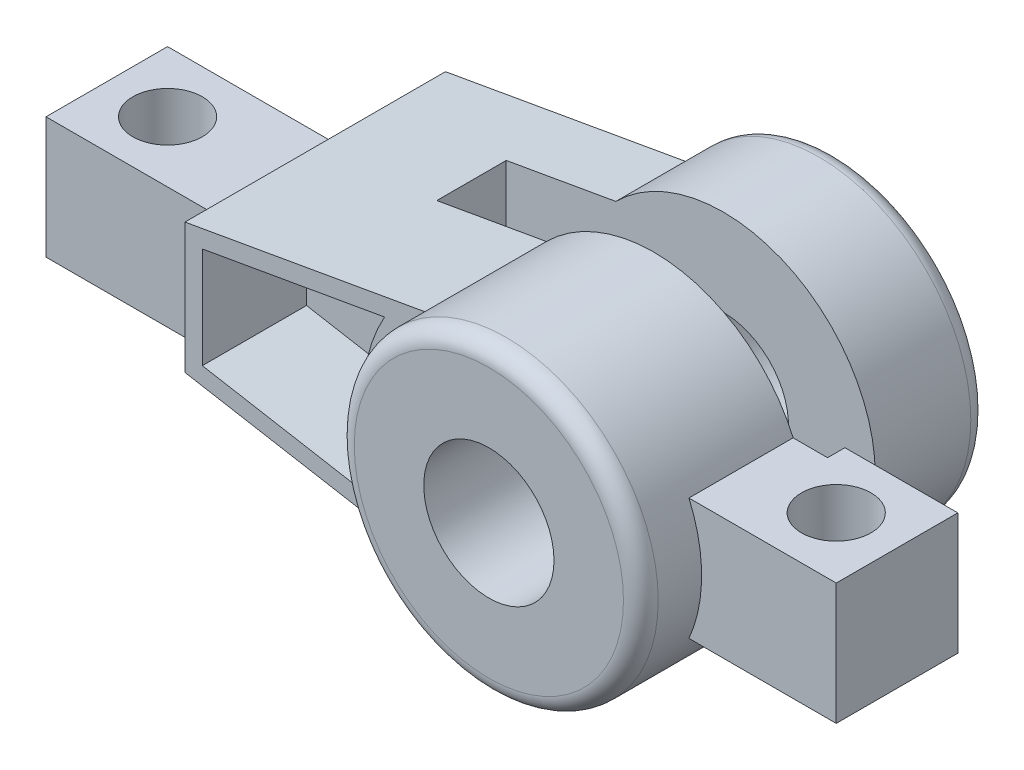
ISO-10303-21;
HEADER;
FILE_DESCRIPTION(('STEP AP214'),'2;1');
FILE_NAME('part.step','',(''),(''),'','','');
FILE_SCHEMA(('AUTOMOTIVE_DESIGN { 1 0 10303 214 1 1 1 1 }'));
ENDSEC;
DATA;
#1=APPLICATION_CONTEXT('core data for automotive mechanical design processes');
#2=APPLICATION_PROTOCOL_DEFINITION('international standard','automotive_design',2000,#1);
#3=PRODUCT_CONTEXT('',#1,'mechanical');
#4=PRODUCT('Part','Part','',(#3));
#5=PRODUCT_RELATED_PRODUCT_CATEGORY('part','',(#4));
#6=PRODUCT_DEFINITION_FORMATION('','',#4);
#7=PRODUCT_DEFINITION_CONTEXT('part definition',#1,'design');
#8=PRODUCT_DEFINITION('design','',#6,#7);
#9=PRODUCT_DEFINITION_SHAPE('','',#8);
#10=(LENGTH_UNIT() NAMED_UNIT(*) SI_UNIT(.MILLI.,.METRE.));
#11=(NAMED_UNIT(*) PLANE_ANGLE_UNIT() SI_UNIT($,.RADIAN.));
#12=(NAMED_UNIT(*) SI_UNIT($,.STERADIAN.) SOLID_ANGLE_UNIT());
#13=UNCERTAINTY_MEASURE_WITH_UNIT(LENGTH_MEASURE(1.E-05),#10,'distance_accuracy_value','');
#14=(GEOMETRIC_REPRESENTATION_CONTEXT(3) GLOBAL_UNCERTAINTY_ASSIGNED_CONTEXT((#13)) GLOBAL_UNIT_ASSIGNED_CONTEXT((#10,
#11,#12)) REPRESENTATION_CONTEXT('',''));
#15=CARTESIAN_POINT('',(0.,0.,0.));
#16=DIRECTION('',(0.,0.,1.));
#17=DIRECTION('',(1.,0.,0.));
#18=AXIS2_PLACEMENT_3D('',#15,#16,#17);
#19=CARTESIAN_POINT('',(46.,-6.99999999999998,20.));
#20=DIRECTION('',(0.,1.,0.));
#21=DIRECTION('',(-1.,0.,0.));
#22=AXIS2_PLACEMENT_3D('',#19,#20,#21);
#23=PLANE('',#22);
#24=CARTESIAN_POINT('',(39.,-6.99999999999998,6.));
#25=DIRECTION('',(0.,1.,0.));
#26=DIRECTION('',(-1.,0.,0.));
#27=AXIS2_PLACEMENT_3D('',#24,#25,#26);
#28=CIRCLE('',#27,5.);
#29=CARTESIAN_POINT('',(34.,-6.99999999999999,6.));
#30=VERTEX_POINT('',#29);
#31=EDGE_CURVE('E11',#30,#30,#28,.T.);
#32=ORIENTED_EDGE('',*,*,#31,.T.);
#33=EDGE_LOOP('',(#32));
#34=FACE_BOUND('',#33,.T.);
#35=DIRECTION('',(-1.,0.,0.));
#36=VECTOR('',#35,1.);
#37=CARTESIAN_POINT('',(46.,-6.99999999999998,-1.));
#38=LINE('',#37,#36);
#39=CARTESIAN_POINT('',(46.,-6.99999999999998,-1.));
#40=VERTEX_POINT('',#39);
#41=CARTESIAN_POINT('',(33.,-6.99999999999999,-1.));
#42=VERTEX_POINT('',#41);
#43=EDGE_CURVE('E293',#40,#42,#38,.T.);
#44=ORIENTED_EDGE('',*,*,#43,.F.);
#45=DIRECTION('',(0.,0.,-1.));
#46=VECTOR('',#45,1.);
#47=CARTESIAN_POINT('',(46.,-6.99999999999998,20.));
#48=LINE('',#47,#46);
#49=CARTESIAN_POINT('',(46.,-6.99999999999998,13.));
#50=VERTEX_POINT('',#49);
#51=EDGE_CURVE('E396',#50,#40,#48,.T.);
#52=ORIENTED_EDGE('',*,*,#51,.F.);
#53=DIRECTION('',(1.,0.,0.));
#54=VECTOR('',#53,1.);
#55=CARTESIAN_POINT('',(29.0390149323454,-6.99999999999998,13.));
#56=LINE('',#55,#54);
#57=CARTESIAN_POINT('',(29.0390149323454,-6.99999999999998,13.));
#58=VERTEX_POINT('',#57);
#59=EDGE_CURVE('E332',#58,#50,#56,.T.);
#60=ORIENTED_EDGE('',*,*,#59,.F.);
#61=DIRECTION('',(0.,0.,-1.));
#62=VECTOR('',#61,1.);
#63=CARTESIAN_POINT('',(29.0390149323454,-6.99999999999998,20.));
#64=LINE('',#63,#62);
#65=CARTESIAN_POINT('',(29.0390149323454,-6.99999999999999,1.));
#66=VERTEX_POINT('',#65);
#67=EDGE_CURVE('E397',#58,#66,#64,.T.);
#68=ORIENTED_EDGE('',*,*,#67,.T.);
#69=DIRECTION('',(1.,0.,0.));
#70=VECTOR('',#69,1.);
#71=CARTESIAN_POINT('',(46.,-6.99999999999998,1.));
#72=LINE('',#71,#70);
#73=CARTESIAN_POINT('',(33.,-6.99999999999999,1.));
#74=VERTEX_POINT('',#73);
#75=EDGE_CURVE('E363',#66,#74,#72,.T.);
#76=ORIENTED_EDGE('',*,*,#75,.T.);
#77=DIRECTION('',(0.,0.,-1.));
#78=VECTOR('',#77,1.);
#79=CARTESIAN_POINT('',(33.,-6.99999999999999,20.));
#80=LINE('',#79,#78);
#81=EDGE_CURVE('E379',#74,#42,#80,.T.);
#82=ORIENTED_EDGE('',*,*,#81,.T.);
#83=EDGE_LOOP('',(#44,#52,#60,#68,#76,#82));
#84=FACE_BOUND('',#83,.T.);
#85=ADVANCED_FACE('F41',(#34,#84),#23,.F.);
#86=CARTESIAN_POINT('',(46.,-6.99999999999998,20.));
#87=DIRECTION('',(-1.,0.,0.));
#88=DIRECTION('',(0.,0.,1.));
#89=AXIS2_PLACEMENT_3D('',#86,#87,#88);
#90=PLANE('',#89);
#91=DIRECTION('',(0.,-1.,0.));
#92=VECTOR('',#91,1.);
#93=CARTESIAN_POINT('',(46.,7.00000000000002,-1.));
#94=LINE('',#93,#92);
#95=CARTESIAN_POINT('',(46.,7.00000000000002,-1.));
#96=VERTEX_POINT('',#95);
#97=EDGE_CURVE('E288',#96,#40,#94,.T.);
#98=ORIENTED_EDGE('',*,*,#97,.F.);
#99=DIRECTION('',(0.,0.,-1.));
#100=VECTOR('',#99,1.);
#101=CARTESIAN_POINT('',(46.,7.00000000000002,20.));
#102=LINE('',#101,#100);
#103=CARTESIAN_POINT('',(46.,7.00000000000002,13.));
#104=VERTEX_POINT('',#103);
#105=EDGE_CURVE('E392',#104,#96,#102,.T.);
#106=ORIENTED_EDGE('',*,*,#105,.F.);
#107=DIRECTION('',(0.,1.,0.));
#108=VECTOR('',#107,1.);
#109=CARTESIAN_POINT('',(46.,-6.99999999999998,13.));
#110=LINE('',#109,#108);
#111=EDGE_CURVE('E340',#50,#104,#110,.T.);
#112=ORIENTED_EDGE('',*,*,#111,.F.);
#113=ORIENTED_EDGE('',*,*,#51,.T.);
#114=EDGE_LOOP('',(#98,#106,#112,#113));
#115=FACE_BOUND('',#114,.T.);
#116=ADVANCED_FACE('F457',(#115),#90,.F.);
#117=CARTESIAN_POINT('',(46.,7.00000000000002,20.));
#118=DIRECTION('',(0.,-1.,0.));
#119=DIRECTION('',(1.,0.,0.));
#120=AXIS2_PLACEMENT_3D('',#117,#118,#119);
#121=PLANE('',#120);
#122=CARTESIAN_POINT('',(39.,7.,6.));
#123=DIRECTION('',(0.,1.,0.));
#124=DIRECTION('',(-1.,0.,0.));
#125=AXIS2_PLACEMENT_3D('',#122,#123,#124);
#126=CIRCLE('',#125,4.);
#127=CARTESIAN_POINT('',(35.,7.,6.));
#128=VERTEX_POINT('',#127);
#129=EDGE_CURVE('E241',#128,#128,#126,.T.);
#130=ORIENTED_EDGE('',*,*,#129,.F.);
#131=EDGE_LOOP('',(#130));
#132=FACE_BOUND('',#131,.T.);
#133=DIRECTION('',(1.,0.,0.));
#134=VECTOR('',#133,1.);
#135=CARTESIAN_POINT('',(29.0390149323454,7.00000000000001,-1.));
#136=LINE('',#135,#134);
#137=CARTESIAN_POINT('',(33.,7.00000000000002,-1.));
#138=VERTEX_POINT('',#137);
#139=EDGE_CURVE('E285',#138,#96,#136,.T.);
#140=ORIENTED_EDGE('',*,*,#139,.F.);
#141=DIRECTION('',(0.,0.,1.));
#142=VECTOR('',#141,1.);
#143=CARTESIAN_POINT('',(33.,7.00000000000002,20.));
#144=LINE('',#143,#142);
#145=CARTESIAN_POINT('',(33.,7.00000000000002,1.));
#146=VERTEX_POINT('',#145);
#147=EDGE_CURVE('E422',#138,#146,#144,.T.);
#148=ORIENTED_EDGE('',*,*,#147,.T.);
#149=DIRECTION('',(-1.,0.,0.));
#150=VECTOR('',#149,1.);
#151=CARTESIAN_POINT('',(46.,7.00000000000002,1.));
#152=LINE('',#151,#150);
#153=CARTESIAN_POINT('',(29.0390149323454,7.00000000000001,1.));
#154=VERTEX_POINT('',#153);
#155=EDGE_CURVE('E351',#146,#154,#152,.T.);
#156=ORIENTED_EDGE('',*,*,#155,.T.);
#157=DIRECTION('',(0.,0.,-1.));
#158=VECTOR('',#157,1.);
#159=CARTESIAN_POINT('',(29.0390149323454,7.00000000000001,20.));
#160=LINE('',#159,#158);
#161=CARTESIAN_POINT('',(29.0390149323454,7.00000000000001,13.));
#162=VERTEX_POINT('',#161);
#163=EDGE_CURVE('E388',#162,#154,#160,.T.);
#164=ORIENTED_EDGE('',*,*,#163,.F.);
#165=DIRECTION('',(-1.,0.,0.));
#166=VECTOR('',#165,1.);
#167=CARTESIAN_POINT('',(46.,7.00000000000002,13.));
#168=LINE('',#167,#166);
#169=EDGE_CURVE('E339',#104,#162,#168,.T.);
#170=ORIENTED_EDGE('',*,*,#169,.F.);
#171=ORIENTED_EDGE('',*,*,#105,.T.);
#172=EDGE_LOOP('',(#140,#148,#156,#164,#170,#171));
#173=FACE_BOUND('',#172,.T.);
#174=ADVANCED_FACE('F467',(#132,#173),#121,.F.);
#175=CARTESIAN_POINT('',(33.,-17.5,-7.));
#176=DIRECTION('',(1.,0.,0.));
#177=DIRECTION('',(0.,0.,-1.));
#178=AXIS2_PLACEMENT_3D('',#175,#176,#177);
#179=PLANE('',#178);
#180=DIRECTION('',(0.,1.,0.));
#181=VECTOR('',#180,1.);
#182=CARTESIAN_POINT('',(33.,-17.5,-1.));
#183=LINE('',#182,#181);
#184=EDGE_CURVE('E431',#42,#138,#183,.T.);
#185=ORIENTED_EDGE('',*,*,#184,.F.);
#186=ORIENTED_EDGE('',*,*,#81,.F.);
#187=DIRECTION('',(0.,1.,0.));
#188=VECTOR('',#187,1.);
#189=CARTESIAN_POINT('',(33.,-17.5,1.));
#190=LINE('',#189,#188);
#191=EDGE_CURVE('E350',#74,#146,#190,.T.);
#192=ORIENTED_EDGE('',*,*,#191,.T.);
#193=ORIENTED_EDGE('',*,*,#147,.F.);
#194=EDGE_LOOP('',(#185,#186,#192,#193));
#195=FACE_BOUND('',#194,.T.);
#196=ADVANCED_FACE('F499',(#195),#179,.F.);
#197=CARTESIAN_POINT('',(-46.,7.,20.));
#198=DIRECTION('',(0.,-1.,0.));
#199=DIRECTION('',(1.,0.,0.));
#200=AXIS2_PLACEMENT_3D('',#197,#198,#199);
#201=PLANE('',#200);
#202=CARTESIAN_POINT('',(-39.,7.,5.));
#203=DIRECTION('',(0.,1.,0.));
#204=DIRECTION('',(-1.,0.,0.));
#205=AXIS2_PLACEMENT_3D('',#202,#203,#204);
#206=CIRCLE('',#205,4.);
#207=CARTESIAN_POINT('',(-43.,7.,5.));
#208=VERTEX_POINT('',#207);
#209=EDGE_CURVE('E944',#208,#208,#206,.T.);
#210=ORIENTED_EDGE('',*,*,#209,.F.);
#211=EDGE_LOOP('',(#210));
#212=FACE_BOUND('',#211,.T.);
#213=DIRECTION('',(-1.,0.,0.));
#214=VECTOR('',#213,1.);
#215=CARTESIAN_POINT('',(-27.,7.,12.));
#216=LINE('',#215,#214);
#217=CARTESIAN_POINT('',(-27.,7.,12.));
#218=VERTEX_POINT('',#217);
#219=CARTESIAN_POINT('',(-46.,7.,12.));
#220=VERTEX_POINT('',#219);
#221=EDGE_CURVE('E294',#218,#220,#216,.T.);
#222=ORIENTED_EDGE('',*,*,#221,.F.);
#223=DIRECTION('',(0.,0.,-1.));
#224=VECTOR('',#223,1.);
#225=CARTESIAN_POINT('',(-27.,7.,20.));
#226=LINE('',#225,#224);
#227=CARTESIAN_POINT('',(-27.,7.,-2.));
#228=VERTEX_POINT('',#227);
#229=EDGE_CURVE('E412',#218,#228,#226,.T.);
#230=ORIENTED_EDGE('',*,*,#229,.T.);
#231=DIRECTION('',(1.,0.,0.));
#232=VECTOR('',#231,1.);
#233=CARTESIAN_POINT('',(-46.,7.,-2.));
#234=LINE('',#233,#232);
#235=CARTESIAN_POINT('',(-46.,7.,-2.));
#236=VERTEX_POINT('',#235);
#237=EDGE_CURVE('E304',#236,#228,#234,.T.);
#238=ORIENTED_EDGE('',*,*,#237,.F.);
#239=DIRECTION('',(0.,0.,-1.));
#240=VECTOR('',#239,1.);
#241=CARTESIAN_POINT('',(-46.,7.,20.));
#242=LINE('',#241,#240);
#243=EDGE_CURVE('E415',#220,#236,#242,.T.);
#244=ORIENTED_EDGE('',*,*,#243,.F.);
#245=EDGE_LOOP('',(#222,#230,#238,#244));
#246=FACE_BOUND('',#245,.T.);
#247=ADVANCED_FACE('F496',(#212,#246),#201,.F.);
#248=CARTESIAN_POINT('',(-46.,-7.,20.));
#249=DIRECTION('',(1.,0.,0.));
#250=DIRECTION('',(0.,0.,-1.));
#251=AXIS2_PLACEMENT_3D('',#248,#249,#250);
#252=PLANE('',#251);
#253=DIRECTION('',(0.,-1.,0.));
#254=VECTOR('',#253,1.);
#255=CARTESIAN_POINT('',(-46.,7.,12.));
#256=LINE('',#255,#254);
#257=CARTESIAN_POINT('',(-46.,-7.,12.));
#258=VERTEX_POINT('',#257);
#259=EDGE_CURVE('E300',#220,#258,#256,.T.);
#260=ORIENTED_EDGE('',*,*,#259,.F.);
#261=ORIENTED_EDGE('',*,*,#243,.T.);
#262=DIRECTION('',(0.,1.,0.));
#263=VECTOR('',#262,1.);
#264=CARTESIAN_POINT('',(-46.,-7.,-2.));
#265=LINE('',#264,#263);
#266=CARTESIAN_POINT('',(-46.,-7.,-2.));
#267=VERTEX_POINT('',#266);
#268=EDGE_CURVE('E305',#267,#236,#265,.T.);
#269=ORIENTED_EDGE('',*,*,#268,.F.);
#270=DIRECTION('',(0.,0.,-1.));
#271=VECTOR('',#270,1.);
#272=CARTESIAN_POINT('',(-46.,-7.,20.));
#273=LINE('',#272,#271);
#274=EDGE_CURVE('E408',#258,#267,#273,.T.);
#275=ORIENTED_EDGE('',*,*,#274,.F.);
#276=EDGE_LOOP('',(#260,#261,#269,#275));
#277=FACE_BOUND('',#276,.T.);
#278=ADVANCED_FACE('F495',(#277),#252,.F.);
#279=CARTESIAN_POINT('',(-46.,-7.,20.));
#280=DIRECTION('',(0.,1.,0.));
#281=DIRECTION('',(-1.,0.,0.));
#282=AXIS2_PLACEMENT_3D('',#279,#280,#281);
#283=PLANE('',#282);
#284=CARTESIAN_POINT('',(-39.,-7.,5.));
#285=DIRECTION('',(0.,1.,0.));
#286=DIRECTION('',(-1.,0.,0.));
#287=AXIS2_PLACEMENT_3D('',#284,#285,#286);
#288=CIRCLE('',#287,4.);
#289=CARTESIAN_POINT('',(-43.,-7.,5.));
#290=VERTEX_POINT('',#289);
#291=EDGE_CURVE('E247',#290,#290,#288,.F.);
#292=ORIENTED_EDGE('',*,*,#291,.F.);
#293=EDGE_LOOP('',(#292));
#294=FACE_BOUND('',#293,.T.);
#295=DIRECTION('',(1.,0.,0.));
#296=VECTOR('',#295,1.);
#297=CARTESIAN_POINT('',(-46.,-7.,12.));
#298=LINE('',#297,#296);
#299=CARTESIAN_POINT('',(-27.,-6.99999999999999,12.));
#300=VERTEX_POINT('',#299);
#301=EDGE_CURVE('E299',#258,#300,#298,.T.);
#302=ORIENTED_EDGE('',*,*,#301,.F.);
#303=ORIENTED_EDGE('',*,*,#274,.T.);
#304=DIRECTION('',(-1.,0.,0.));
#305=VECTOR('',#304,1.);
#306=CARTESIAN_POINT('',(-27.,-6.99999999999999,-2.));
#307=LINE('',#306,#305);
#308=CARTESIAN_POINT('',(-27.,-6.99999999999999,-2.));
#309=VERTEX_POINT('',#308);
#310=EDGE_CURVE('E311',#309,#267,#307,.T.);
#311=ORIENTED_EDGE('',*,*,#310,.F.);
#312=DIRECTION('',(0.,0.,-1.));
#313=VECTOR('',#312,1.);
#314=CARTESIAN_POINT('',(-27.,-6.99999999999999,20.));
#315=LINE('',#314,#313);
#316=EDGE_CURVE('E409',#300,#309,#315,.T.);
#317=ORIENTED_EDGE('',*,*,#316,.F.);
#318=EDGE_LOOP('',(#302,#303,#311,#317));
#319=FACE_BOUND('',#318,.T.);
#320=ADVANCED_FACE('F490',(#294,#319),#283,.F.);
#321=CARTESIAN_POINT('',(-27.,7.5,20.));
#322=DIRECTION('',(0.173648177666928,-0.984807753012209,0.));
#323=DIRECTION('',(0.984807753012209,0.173648177666928,0.));
#324=AXIS2_PLACEMENT_3D('',#321,#322,#323);
#325=PLANE('',#324);
#326=DIRECTION('',(0.984807753012209,0.173648177666928,0.));
#327=VECTOR('',#326,1.);
#328=CARTESIAN_POINT('',(0.621718040461723,12.3704541440551,-15.));
#329=LINE('',#328,#327);
#330=CARTESIAN_POINT('',(-27.,7.5,-15.));
#331=VERTEX_POINT('',#330);
#332=CARTESIAN_POINT('',(0.621718040461723,12.3704541440551,-15.));
#333=VERTEX_POINT('',#332);
#334=EDGE_CURVE('E322',#331,#333,#329,.T.);
#335=ORIENTED_EDGE('',*,*,#334,.F.);
#336=DIRECTION('',(0.,0.,-1.));
#337=VECTOR('',#336,1.);
#338=CARTESIAN_POINT('',(-27.,7.5,20.));
#339=LINE('',#338,#337);
#340=CARTESIAN_POINT('',(-27.,7.5,15.));
#341=VERTEX_POINT('',#340);
#342=EDGE_CURVE('E419',#341,#331,#339,.T.);
#343=ORIENTED_EDGE('',*,*,#342,.F.);
#344=DIRECTION('',(-0.984807753012209,-0.173648177666928,0.));
#345=VECTOR('',#344,1.);
#346=CARTESIAN_POINT('',(-2.09672515686145,11.8911192628436,15.));
#347=LINE('',#346,#345);
#348=CARTESIAN_POINT('',(0.621718040461722,12.3704541440551,15.));
#349=VERTEX_POINT('',#348);
#350=EDGE_CURVE('E326',#349,#341,#347,.T.);
#351=ORIENTED_EDGE('',*,*,#350,.F.);
#352=DIRECTION('',(0.,0.,-1.));
#353=VECTOR('',#352,1.);
#354=CARTESIAN_POINT('',(0.621718040461723,12.3704541440551,20.));
#355=LINE('',#354,#353);
#356=CARTESIAN_POINT('',(0.621718040461723,12.3704541440551,1.));
#357=VERTEX_POINT('',#356);
#358=EDGE_CURVE('E417',#349,#357,#355,.T.);
#359=ORIENTED_EDGE('',*,*,#358,.T.);
#360=DIRECTION('',(-0.984807753012209,-0.173648177666928,0.));
#361=VECTOR('',#360,1.);
#362=CARTESIAN_POINT('',(-27.,7.5,1.));
#363=LINE('',#362,#361);
#364=CARTESIAN_POINT('',(-12.,10.1449047106269,1.));
#365=VERTEX_POINT('',#364);
#366=EDGE_CURVE('E356',#357,#365,#363,.T.);
#367=ORIENTED_EDGE('',*,*,#366,.T.);
#368=DIRECTION('',(0.,0.,-1.));
#369=VECTOR('',#368,1.);
#370=CARTESIAN_POINT('',(-12.,10.1449047106269,20.));
#371=LINE('',#370,#369);
#372=CARTESIAN_POINT('',(-12.,10.1449047106269,-7.));
#373=VERTEX_POINT('',#372);
#374=EDGE_CURVE('E384',#365,#373,#371,.T.);
#375=ORIENTED_EDGE('',*,*,#374,.T.);
#376=DIRECTION('',(0.984807753012209,0.173648177666928,0.));
#377=VECTOR('',#376,1.);
#378=CARTESIAN_POINT('',(-27.,7.5,-7.));
#379=LINE('',#378,#377);
#380=CARTESIAN_POINT('',(0.621718040461723,12.3704541440551,-7.));
#381=VERTEX_POINT('',#380);
#382=EDGE_CURVE('E371',#373,#381,#379,.T.);
#383=ORIENTED_EDGE('',*,*,#382,.T.);
#384=EDGE_CURVE('E418',#381,#333,#355,.T.);
#385=ORIENTED_EDGE('',*,*,#384,.T.);
#386=EDGE_LOOP('',(#335,#343,#351,#359,#367,#375,#383,#385));
#387=FACE_BOUND('',#386,.T.);
#388=ADVANCED_FACE('F487',(#387),#325,.F.);
#389=CARTESIAN_POINT('',(-27.,-6.99999999999999,20.));
#390=DIRECTION('',(1.,0.,0.));
#391=DIRECTION('',(0.,0.,-1.));
#392=AXIS2_PLACEMENT_3D('',#389,#390,#391);
#393=PLANE('',#392);
#394=DIRECTION('',(0.,1.,0.));
#395=VECTOR('',#394,1.);
#396=CARTESIAN_POINT('',(-27.,-6.99999999999999,12.));
#397=LINE('',#396,#395);
#398=EDGE_CURVE('E291',#300,#218,#397,.T.);
#399=ORIENTED_EDGE('',*,*,#398,.F.);
#400=ORIENTED_EDGE('',*,*,#316,.T.);
#401=DIRECTION('',(0.,-1.,0.));
#402=VECTOR('',#401,1.);
#403=CARTESIAN_POINT('',(-27.,7.,-2.));
#404=LINE('',#403,#402);
#405=EDGE_CURVE('E308',#228,#309,#404,.T.);
#406=ORIENTED_EDGE('',*,*,#405,.F.);
#407=ORIENTED_EDGE('',*,*,#229,.F.);
#408=EDGE_LOOP('',(#399,#400,#406,#407));
#409=FACE_BOUND('',#408,.T.);
#410=ORIENTED_EDGE('',*,*,#342,.T.);
#411=DIRECTION('',(0.,1.,0.));
#412=VECTOR('',#411,1.);
#413=CARTESIAN_POINT('',(-27.,7.5,-15.));
#414=LINE('',#413,#412);
#415=CARTESIAN_POINT('',(-27.,-7.49999999999999,-15.));
#416=VERTEX_POINT('',#415);
#417=EDGE_CURVE('E316',#416,#331,#414,.T.);
#418=ORIENTED_EDGE('',*,*,#417,.F.);
#419=DIRECTION('',(0.,0.,-1.));
#420=VECTOR('',#419,1.);
#421=CARTESIAN_POINT('',(-27.,-7.49999999999999,20.));
#422=LINE('',#421,#420);
#423=CARTESIAN_POINT('',(-27.,-7.49999999999999,15.));
#424=VERTEX_POINT('',#423);
#425=EDGE_CURVE('E403',#424,#416,#422,.T.);
#426=ORIENTED_EDGE('',*,*,#425,.F.);
#427=DIRECTION('',(0.,-1.,0.));
#428=VECTOR('',#427,1.);
#429=CARTESIAN_POINT('',(-27.,0.,15.));
#430=LINE('',#429,#428);
#431=EDGE_CURVE('E328',#341,#424,#430,.T.);
#432=ORIENTED_EDGE('',*,*,#431,.F.);
#433=EDGE_LOOP('',(#410,#418,#426,#432));
#434=FACE_BOUND('',#433,.T.);
#435=ADVANCED_FACE('F485',(#409,#434),#393,.F.);
#436=CARTESIAN_POINT('',(-27.,-7.49999999999999,20.));
#437=DIRECTION('',(0.173648177666927,0.984807753012209,0.));
#438=DIRECTION('',(-0.984807753012209,0.173648177666927,0.));
#439=AXIS2_PLACEMENT_3D('',#436,#437,#438);
#440=PLANE('',#439);
#441=DIRECTION('',(-0.984807753012209,0.173648177666927,0.));
#442=VECTOR('',#441,1.);
#443=CARTESIAN_POINT('',(-27.,-7.49999999999999,-15.));
#444=LINE('',#443,#442);
#445=CARTESIAN_POINT('',(0.621718040461723,-12.3704541440551,-15.));
#446=VERTEX_POINT('',#445);
#447=EDGE_CURVE('E317',#446,#416,#444,.T.);
#448=ORIENTED_EDGE('',*,*,#447,.F.);
#449=DIRECTION('',(0.,0.,-1.));
#450=VECTOR('',#449,1.);
#451=CARTESIAN_POINT('',(0.621718040461723,-12.3704541440551,20.));
#452=LINE('',#451,#450);
#453=CARTESIAN_POINT('',(0.621718040461719,-12.3704541440551,-7.));
#454=VERTEX_POINT('',#453);
#455=EDGE_CURVE('E405',#454,#446,#452,.T.);
#456=ORIENTED_EDGE('',*,*,#455,.F.);
#457=DIRECTION('',(-0.984807753012209,0.173648177666927,0.));
#458=VECTOR('',#457,1.);
#459=CARTESIAN_POINT('',(-27.,-7.49999999999999,-7.));
#460=LINE('',#459,#458);
#461=CARTESIAN_POINT('',(-12.,-10.1449047106269,-7.));
#462=VERTEX_POINT('',#461);
#463=EDGE_CURVE('E380',#454,#462,#460,.T.);
#464=ORIENTED_EDGE('',*,*,#463,.T.);
#465=DIRECTION('',(0.,0.,1.));
#466=VECTOR('',#465,1.);
#467=CARTESIAN_POINT('',(-12.,-10.1449047106269,20.));
#468=LINE('',#467,#466);
#469=CARTESIAN_POINT('',(-12.,-10.1449047106269,1.));
#470=VERTEX_POINT('',#469);
#471=EDGE_CURVE('E426',#462,#470,#468,.T.);
#472=ORIENTED_EDGE('',*,*,#471,.T.);
#473=DIRECTION('',(0.984807753012209,-0.173648177666927,0.));
#474=VECTOR('',#473,1.);
#475=CARTESIAN_POINT('',(-27.,-7.49999999999999,1.));
#476=LINE('',#475,#474);
#477=CARTESIAN_POINT('',(0.621718040461719,-12.3704541440551,1.));
#478=VERTEX_POINT('',#477);
#479=EDGE_CURVE('E370',#470,#478,#476,.T.);
#480=ORIENTED_EDGE('',*,*,#479,.T.);
#481=CARTESIAN_POINT('',(0.621718040461711,-12.3704541440551,15.));
#482=VERTEX_POINT('',#481);
#483=EDGE_CURVE('E401',#482,#478,#452,.T.);
#484=ORIENTED_EDGE('',*,*,#483,.F.);
#485=DIRECTION('',(0.984807753012209,-0.173648177666927,0.));
#486=VECTOR('',#485,1.);
#487=CARTESIAN_POINT('',(-2.09672515686144,-11.8911192628436,15.));
#488=LINE('',#487,#486);
#489=EDGE_CURVE('E329',#424,#482,#488,.T.);
#490=ORIENTED_EDGE('',*,*,#489,.F.);
#491=ORIENTED_EDGE('',*,*,#425,.T.);
#492=EDGE_LOOP('',(#448,#456,#464,#472,#480,#484,#490,#491));
#493=FACE_BOUND('',#492,.T.);
#494=ADVANCED_FACE('F477',(#493),#440,.F.);
#495=CARTESIAN_POINT('',(13.,0.,-20.));
#496=DIRECTION('',(0.,0.,1.));
#497=DIRECTION('',(1.,0.,0.));
#498=AXIS2_PLACEMENT_3D('',#495,#496,#497);
#499=PLANE('',#498);
#500=CARTESIAN_POINT('',(13.,0.,-20.));
#501=DIRECTION('',(0.,0.,1.));
#502=DIRECTION('',(1.,0.,0.));
#503=AXIS2_PLACEMENT_3D('',#500,#501,#502);
#504=CIRCLE('',#503,15.5);
#505=CARTESIAN_POINT('',(28.5,0.,-20.));
#506=VERTEX_POINT('',#505);
#507=EDGE_CURVE('E445',#506,#506,#504,.F.);
#508=ORIENTED_EDGE('',*,*,#507,.T.);
#509=EDGE_LOOP('',(#508));
#510=FACE_BOUND('',#509,.T.);
#511=CARTESIAN_POINT('',(13.,0.,-20.));
#512=DIRECTION('',(0.,0.,1.));
#513=DIRECTION('',(1.,0.,0.));
#514=AXIS2_PLACEMENT_3D('',#511,#512,#513);
#515=CIRCLE('',#514,7.5);
#516=CARTESIAN_POINT('',(20.5,0.,-20.));
#517=VERTEX_POINT('',#516);
#518=EDGE_CURVE('E387',#517,#517,#515,.T.);
#519=ORIENTED_EDGE('',*,*,#518,.T.);
#520=EDGE_LOOP('',(#519));
#521=FACE_BOUND('',#520,.T.);
#522=ADVANCED_FACE('F481',(#510,#521),#499,.F.);
#523=CARTESIAN_POINT('',(13.,0.,20.));
#524=DIRECTION('',(0.,0.,1.));
#525=DIRECTION('',(1.,0.,0.));
#526=AXIS2_PLACEMENT_3D('',#523,#524,#525);
#527=PLANE('',#526);
#528=CARTESIAN_POINT('',(13.,0.,20.));
#529=DIRECTION('',(0.,0.,1.));
#530=DIRECTION('',(1.,0.,0.));
#531=AXIS2_PLACEMENT_3D('',#528,#529,#530);
#532=CIRCLE('',#531,15.5);
#533=CARTESIAN_POINT('',(28.5,0.,20.));
#534=VERTEX_POINT('',#533);
#535=EDGE_CURVE('E433',#534,#534,#532,.T.);
#536=ORIENTED_EDGE('',*,*,#535,.T.);
#537=EDGE_LOOP('',(#536));
#538=FACE_BOUND('',#537,.T.);
#539=CARTESIAN_POINT('',(13.,0.,20.));
#540=DIRECTION('',(0.,0.,1.));
#541=DIRECTION('',(1.,0.,0.));
#542=AXIS2_PLACEMENT_3D('',#539,#540,#541);
#543=CIRCLE('',#542,7.5);
#544=CARTESIAN_POINT('',(20.5,0.,20.));
#545=VERTEX_POINT('',#544);
#546=EDGE_CURVE('E390',#545,#545,#543,.T.);
#547=ORIENTED_EDGE('',*,*,#546,.F.);
#548=EDGE_LOOP('',(#547));
#549=FACE_BOUND('',#548,.T.);
#550=ADVANCED_FACE('F583',(#538,#549),#527,.T.);
#551=CARTESIAN_POINT('',(13.,0.,20.));
#552=DIRECTION('',(0.,0.,-1.));
#553=DIRECTION('',(-1.,0.,0.));
#554=AXIS2_PLACEMENT_3D('',#551,#552,#553);
#555=CYLINDRICAL_SURFACE('',#554,17.5);
#556=CARTESIAN_POINT('',(13.,0.,18.));
#557=DIRECTION('',(0.,0.,1.));
#558=DIRECTION('',(1.,0.,0.));
#559=AXIS2_PLACEMENT_3D('',#556,#557,#558);
#560=CIRCLE('',#559,17.5);
#561=CARTESIAN_POINT('',(30.5,0.,18.));
#562=VERTEX_POINT('',#561);
#563=EDGE_CURVE('E436',#562,#562,#560,.F.);
#564=ORIENTED_EDGE('',*,*,#563,.T.);
#565=EDGE_LOOP('',(#564));
#566=FACE_BOUND('',#565,.T.);
#567=ORIENTED_EDGE('',*,*,#358,.F.);
#568=CARTESIAN_POINT('',(13.,0.,15.));
#569=DIRECTION('',(0.,0.,1.));
#570=DIRECTION('',(1.,0.,0.));
#571=AXIS2_PLACEMENT_3D('',#568,#569,#570);
#572=CIRCLE('',#571,17.5);
#573=EDGE_CURVE('E321',#349,#482,#572,.T.);
#574=ORIENTED_EDGE('',*,*,#573,.T.);
#575=ORIENTED_EDGE('',*,*,#483,.T.);
#576=CARTESIAN_POINT('',(13.,0.,1.));
#577=DIRECTION('',(0.,0.,1.));
#578=DIRECTION('',(1.,0.,0.));
#579=AXIS2_PLACEMENT_3D('',#576,#577,#578);
#580=CIRCLE('',#579,17.5);
#581=EDGE_CURVE('E364',#478,#66,#580,.T.);
#582=ORIENTED_EDGE('',*,*,#581,.T.);
#583=ORIENTED_EDGE('',*,*,#67,.F.);
#584=CARTESIAN_POINT('',(13.,0.,13.));
#585=DIRECTION('',(0.,0.,-1.));
#586=DIRECTION('',(1.,0.,0.));
#587=AXIS2_PLACEMENT_3D('',#584,#585,#586);
#588=CIRCLE('',#587,17.5);
#589=EDGE_CURVE('E335',#162,#58,#588,.T.);
#590=ORIENTED_EDGE('',*,*,#589,.F.);
#591=ORIENTED_EDGE('',*,*,#163,.T.);
#592=CARTESIAN_POINT('',(13.,0.,1.));
#593=DIRECTION('',(0.,0.,1.));
#594=DIRECTION('',(1.,0.,0.));
#595=AXIS2_PLACEMENT_3D('',#592,#593,#594);
#596=CIRCLE('',#595,17.5);
#597=EDGE_CURVE('E352',#154,#357,#596,.T.);
#598=ORIENTED_EDGE('',*,*,#597,.T.);
#599=EDGE_LOOP('',(#567,#574,#575,#582,#583,#590,#591,#598));
#600=FACE_BOUND('',#599,.T.);
#601=ADVANCED_FACE('F478',(#566,#600),#555,.T.);
#602=CARTESIAN_POINT('',(13.,0.,20.));
#603=DIRECTION('',(0.,0.,-1.));
#604=DIRECTION('',(-1.,0.,0.));
#605=AXIS2_PLACEMENT_3D('',#602,#603,#604);
#606=CYLINDRICAL_SURFACE('',#605,7.5);
#607=CARTESIAN_POINT('',(13.,0.,-7.));
#608=DIRECTION('',(0.,0.,-1.));
#609=DIRECTION('',(-1.,0.,0.));
#610=AXIS2_PLACEMENT_3D('',#607,#608,#609);
#611=CIRCLE('',#610,7.5);
#612=CARTESIAN_POINT('',(5.5,0.,-7.));
#613=VERTEX_POINT('',#612);
#614=EDGE_CURVE('E369',#613,#613,#611,.T.);
#615=ORIENTED_EDGE('',*,*,#614,.F.);
#616=EDGE_LOOP('',(#615));
#617=FACE_BOUND('',#616,.T.);
#618=ORIENTED_EDGE('',*,*,#518,.F.);
#619=EDGE_LOOP('',(#618));
#620=FACE_BOUND('',#619,.T.);
#621=ADVANCED_FACE('F476',(#617,#620),#606,.F.);
#622=CARTESIAN_POINT('',(13.,0.,-18.));
#623=DIRECTION('',(0.,0.,1.));
#624=DIRECTION('',(1.,0.,0.));
#625=AXIS2_PLACEMENT_3D('',#622,#623,#624);
#626=CIRCLE('',#625,17.5);
#627=CARTESIAN_POINT('',(30.5,0.,-18.));
#628=VERTEX_POINT('',#627);
#629=EDGE_CURVE('E437',#628,#628,#626,.T.);
#630=ORIENTED_EDGE('',*,*,#629,.T.);
#631=EDGE_LOOP('',(#630));
#632=FACE_BOUND('',#631,.T.);
#633=ORIENTED_EDGE('',*,*,#384,.F.);
#634=CARTESIAN_POINT('',(13.,0.,-7.));
#635=DIRECTION('',(0.,0.,-1.));
#636=DIRECTION('',(-1.,0.,0.));
#637=AXIS2_PLACEMENT_3D('',#634,#635,#636);
#638=CIRCLE('',#637,17.5);
#639=EDGE_CURVE('E372',#381,#454,#638,.T.);
#640=ORIENTED_EDGE('',*,*,#639,.T.);
#641=ORIENTED_EDGE('',*,*,#455,.T.);
#642=CARTESIAN_POINT('',(13.,0.,-15.));
#643=DIRECTION('',(0.,0.,1.));
#644=DIRECTION('',(-1.,0.,0.));
#645=AXIS2_PLACEMENT_3D('',#642,#643,#644);
#646=CIRCLE('',#645,17.5);
#647=EDGE_CURVE('E313',#333,#446,#646,.T.);
#648=ORIENTED_EDGE('',*,*,#647,.F.);
#649=EDGE_LOOP('',(#633,#640,#641,#648));
#650=FACE_BOUND('',#649,.T.);
#651=ADVANCED_FACE('F475',(#632,#650),#555,.T.);
#652=CARTESIAN_POINT('',(13.,0.,1.));
#653=DIRECTION('',(0.,0.,1.));
#654=DIRECTION('',(1.,0.,0.));
#655=AXIS2_PLACEMENT_3D('',#652,#653,#654);
#656=CIRCLE('',#655,7.5);
#657=CARTESIAN_POINT('',(20.5,0.,1.));
#658=VERTEX_POINT('',#657);
#659=EDGE_CURVE('E346',#658,#658,#656,.T.);
#660=ORIENTED_EDGE('',*,*,#659,.F.);
#661=EDGE_LOOP('',(#660));
#662=FACE_BOUND('',#661,.T.);
#663=ORIENTED_EDGE('',*,*,#546,.T.);
#664=EDGE_LOOP('',(#663));
#665=FACE_BOUND('',#664,.T.);
#666=ADVANCED_FACE('F473',(#662,#665),#606,.F.);
#667=CARTESIAN_POINT('',(-12.,-17.5,-7.));
#668=DIRECTION('',(-1.,0.,0.));
#669=DIRECTION('',(0.,0.,1.));
#670=AXIS2_PLACEMENT_3D('',#667,#668,#669);
#671=PLANE('',#670);
#672=DIRECTION('',(0.,1.,0.));
#673=VECTOR('',#672,1.);
#674=CARTESIAN_POINT('',(-12.,-17.5,1.));
#675=LINE('',#674,#673);
#676=EDGE_CURVE('E345',#470,#365,#675,.T.);
#677=ORIENTED_EDGE('',*,*,#676,.F.);
#678=ORIENTED_EDGE('',*,*,#471,.F.);
#679=DIRECTION('',(0.,1.,0.));
#680=VECTOR('',#679,1.);
#681=CARTESIAN_POINT('',(-12.,-17.5,-7.));
#682=LINE('',#681,#680);
#683=EDGE_CURVE('E344',#462,#373,#682,.T.);
#684=ORIENTED_EDGE('',*,*,#683,.T.);
#685=ORIENTED_EDGE('',*,*,#374,.F.);
#686=EDGE_LOOP('',(#677,#678,#684,#685));
#687=FACE_BOUND('',#686,.T.);
#688=ADVANCED_FACE('F532',(#687),#671,.F.);
#689=CARTESIAN_POINT('',(-12.,-17.5,-7.));
#690=DIRECTION('',(0.,0.,-1.));
#691=DIRECTION('',(-1.,0.,0.));
#692=AXIS2_PLACEMENT_3D('',#689,#690,#691);
#693=PLANE('',#692);
#694=ORIENTED_EDGE('',*,*,#614,.T.);
#695=EDGE_LOOP('',(#694));
#696=FACE_BOUND('',#695,.T.);
#697=ORIENTED_EDGE('',*,*,#639,.F.);
#698=ORIENTED_EDGE('',*,*,#382,.F.);
#699=ORIENTED_EDGE('',*,*,#683,.F.);
#700=ORIENTED_EDGE('',*,*,#463,.F.);
#701=EDGE_LOOP('',(#697,#698,#699,#700));
#702=FACE_BOUND('',#701,.T.);
#703=ADVANCED_FACE('F530',(#696,#702),#693,.F.);
#704=CARTESIAN_POINT('',(-12.,-17.5,1.));
#705=DIRECTION('',(0.,0.,1.));
#706=DIRECTION('',(1.,0.,0.));
#707=AXIS2_PLACEMENT_3D('',#704,#705,#706);
#708=PLANE('',#707);
#709=ORIENTED_EDGE('',*,*,#659,.T.);
#710=EDGE_LOOP('',(#709));
#711=FACE_BOUND('',#710,.T.);
#712=ORIENTED_EDGE('',*,*,#676,.T.);
#713=ORIENTED_EDGE('',*,*,#366,.F.);
#714=ORIENTED_EDGE('',*,*,#597,.F.);
#715=ORIENTED_EDGE('',*,*,#155,.F.);
#716=ORIENTED_EDGE('',*,*,#191,.F.);
#717=ORIENTED_EDGE('',*,*,#75,.F.);
#718=ORIENTED_EDGE('',*,*,#581,.F.);
#719=ORIENTED_EDGE('',*,*,#479,.F.);
#720=EDGE_LOOP('',(#712,#713,#714,#715,#716,#717,#718,#719));
#721=FACE_BOUND('',#720,.T.);
#722=ADVANCED_FACE('F548',(#711,#721),#708,.F.);
#723=CARTESIAN_POINT('',(13.,0.,13.));
#724=DIRECTION('',(0.,0.,1.));
#725=DIRECTION('',(1.,0.,0.));
#726=AXIS2_PLACEMENT_3D('',#723,#724,#725);
#727=PLANE('',#726);
#728=ORIENTED_EDGE('',*,*,#589,.T.);
#729=ORIENTED_EDGE('',*,*,#59,.T.);
#730=ORIENTED_EDGE('',*,*,#111,.T.);
#731=ORIENTED_EDGE('',*,*,#169,.T.);
#732=EDGE_LOOP('',(#728,#729,#730,#731));
#733=FACE_BOUND('',#732,.T.);
#734=ADVANCED_FACE('F554',(#733),#727,.T.);
#735=CARTESIAN_POINT('',(0.,0.,15.));
#736=DIRECTION('',(0.,0.,1.));
#737=DIRECTION('',(1.,0.,0.));
#738=AXIS2_PLACEMENT_3D('',#735,#736,#737);
#739=PLANE('',#738);
#740=CARTESIAN_POINT('',(13.,0.,15.));
#741=DIRECTION('',(0.,0.,-1.));
#742=DIRECTION('',(1.,0.,0.));
#743=AXIS2_PLACEMENT_3D('',#740,#741,#742);
#744=CIRCLE('',#743,19.5000000000002);
#745=CARTESIAN_POINT('',(-4.0173101960299,-9.5216150779217,15.));
#746=VERTEX_POINT('',#745);
#747=CARTESIAN_POINT('',(-4.01731019602989,9.52161507792171,15.));
#748=VERTEX_POINT('',#747);
#749=EDGE_CURVE('E63',#746,#748,#744,.T.);
#750=ORIENTED_EDGE('',*,*,#749,.F.);
#751=DIRECTION('',(0.984807753012209,-0.173648177666927,0.));
#752=VECTOR('',#751,1.);
#753=CARTESIAN_POINT('',(-25.,-5.82180073764543,15.));
#754=LINE('',#753,#752);
#755=CARTESIAN_POINT('',(-25.,-5.82180073764543,15.));
#756=VERTEX_POINT('',#755);
#757=EDGE_CURVE('E261',#756,#746,#754,.T.);
#758=ORIENTED_EDGE('',*,*,#757,.F.);
#759=DIRECTION('',(0.,-1.,0.));
#760=VECTOR('',#759,1.);
#761=CARTESIAN_POINT('',(-25.,5.82180073764543,15.));
#762=LINE('',#761,#760);
#763=CARTESIAN_POINT('',(-25.,5.82180073764543,15.));
#764=VERTEX_POINT('',#763);
#765=EDGE_CURVE('E273',#764,#756,#762,.T.);
#766=ORIENTED_EDGE('',*,*,#765,.F.);
#767=DIRECTION('',(-0.984807753012209,-0.173648177666927,0.));
#768=VECTOR('',#767,1.);
#769=CARTESIAN_POINT('',(-4.01731019602989,9.52161507792171,15.));
#770=LINE('',#769,#768);
#771=EDGE_CURVE('E275',#748,#764,#770,.T.);
#772=ORIENTED_EDGE('',*,*,#771,.F.);
#773=EDGE_LOOP('',(#750,#758,#766,#772));
#774=FACE_BOUND('',#773,.T.);
#775=ORIENTED_EDGE('',*,*,#573,.F.);
#776=ORIENTED_EDGE('',*,*,#350,.T.);
#777=ORIENTED_EDGE('',*,*,#431,.T.);
#778=ORIENTED_EDGE('',*,*,#489,.T.);
#779=EDGE_LOOP('',(#775,#776,#777,#778));
#780=FACE_BOUND('',#779,.T.);
#781=ADVANCED_FACE('F551',(#774,#780),#739,.T.);
#782=CARTESIAN_POINT('',(13.,0.,-15.));
#783=DIRECTION('',(0.,0.,-1.));
#784=DIRECTION('',(-1.,0.,0.));
#785=AXIS2_PLACEMENT_3D('',#782,#783,#784);
#786=PLANE('',#785);
#787=CARTESIAN_POINT('',(13.,0.,-15.));
#788=DIRECTION('',(0.,0.,1.));
#789=DIRECTION('',(-1.,0.,0.));
#790=AXIS2_PLACEMENT_3D('',#787,#788,#789);
#791=CIRCLE('',#790,19.5000000000002);
#792=CARTESIAN_POINT('',(-4.01731019602988,9.52161507792171,-15.));
#793=VERTEX_POINT('',#792);
#794=CARTESIAN_POINT('',(-4.01731019602989,-9.5216150779217,-15.));
#795=VERTEX_POINT('',#794);
#796=EDGE_CURVE('E60',#793,#795,#791,.T.);
#797=ORIENTED_EDGE('',*,*,#796,.F.);
#798=DIRECTION('',(0.984807753012209,0.173648177666928,0.));
#799=VECTOR('',#798,1.);
#800=CARTESIAN_POINT('',(-25.,5.82180073764543,-15.));
#801=LINE('',#800,#799);
#802=CARTESIAN_POINT('',(-25.,5.82180073764543,-15.));
#803=VERTEX_POINT('',#802);
#804=EDGE_CURVE('E232',#803,#793,#801,.T.);
#805=ORIENTED_EDGE('',*,*,#804,.F.);
#806=DIRECTION('',(0.,1.,0.));
#807=VECTOR('',#806,1.);
#808=CARTESIAN_POINT('',(-25.,-5.82180073764543,-15.));
#809=LINE('',#808,#807);
#810=CARTESIAN_POINT('',(-25.,-5.82180073764543,-15.));
#811=VERTEX_POINT('',#810);
#812=EDGE_CURVE('E238',#811,#803,#809,.T.);
#813=ORIENTED_EDGE('',*,*,#812,.F.);
#814=DIRECTION('',(-0.984807753012209,0.173648177666927,0.));
#815=VECTOR('',#814,1.);
#816=CARTESIAN_POINT('',(-4.01731019602989,-9.5216150779217,-15.));
#817=LINE('',#816,#815);
#818=EDGE_CURVE('E250',#795,#811,#817,.T.);
#819=ORIENTED_EDGE('',*,*,#818,.F.);
#820=EDGE_LOOP('',(#797,#805,#813,#819));
#821=FACE_BOUND('',#820,.T.);
#822=ORIENTED_EDGE('',*,*,#647,.T.);
#823=ORIENTED_EDGE('',*,*,#447,.T.);
#824=ORIENTED_EDGE('',*,*,#417,.T.);
#825=ORIENTED_EDGE('',*,*,#334,.T.);
#826=EDGE_LOOP('',(#822,#823,#824,#825));
#827=FACE_BOUND('',#826,.T.);
#828=ADVANCED_FACE('F540',(#821,#827),#786,.T.);
#829=CARTESIAN_POINT('',(0.,0.,-2.));
#830=DIRECTION('',(0.,0.,-1.));
#831=DIRECTION('',(-1.,0.,0.));
#832=AXIS2_PLACEMENT_3D('',#829,#830,#831);
#833=PLANE('',#832);
#834=ORIENTED_EDGE('',*,*,#268,.T.);
#835=ORIENTED_EDGE('',*,*,#237,.T.);
#836=ORIENTED_EDGE('',*,*,#405,.T.);
#837=ORIENTED_EDGE('',*,*,#310,.T.);
#838=EDGE_LOOP('',(#834,#835,#836,#837));
#839=FACE_BOUND('',#838,.T.);
#840=ADVANCED_FACE('F563',(#839),#833,.T.);
#841=CARTESIAN_POINT('',(0.,0.,12.));
#842=DIRECTION('',(0.,0.,1.));
#843=DIRECTION('',(1.,0.,0.));
#844=AXIS2_PLACEMENT_3D('',#841,#842,#843);
#845=PLANE('',#844);
#846=ORIENTED_EDGE('',*,*,#398,.T.);
#847=ORIENTED_EDGE('',*,*,#221,.T.);
#848=ORIENTED_EDGE('',*,*,#259,.T.);
#849=ORIENTED_EDGE('',*,*,#301,.T.);
#850=EDGE_LOOP('',(#846,#847,#848,#849));
#851=FACE_BOUND('',#850,.T.);
#852=ADVANCED_FACE('F614',(#851),#845,.T.);
#853=CARTESIAN_POINT('',(13.,0.,-1.));
#854=DIRECTION('',(0.,0.,-1.));
#855=DIRECTION('',(-1.,0.,0.));
#856=AXIS2_PLACEMENT_3D('',#853,#854,#855);
#857=PLANE('',#856);
#858=ORIENTED_EDGE('',*,*,#184,.T.);
#859=ORIENTED_EDGE('',*,*,#139,.T.);
#860=ORIENTED_EDGE('',*,*,#97,.T.);
#861=ORIENTED_EDGE('',*,*,#43,.T.);
#862=EDGE_LOOP('',(#858,#859,#860,#861));
#863=FACE_BOUND('',#862,.T.);
#864=ADVANCED_FACE('F608',(#863),#857,.T.);
#865=CARTESIAN_POINT('',(13.,0.,3.));
#866=DIRECTION('',(0.,0.,1.));
#867=DIRECTION('',(1.,0.,0.));
#868=AXIS2_PLACEMENT_3D('',#865,#866,#867);
#869=CYLINDRICAL_SURFACE('',#868,19.5000000000002);
#870=ORIENTED_EDGE('',*,*,#749,.T.);
#871=DIRECTION('',(0.,0.,1.));
#872=VECTOR('',#871,1.);
#873=CARTESIAN_POINT('',(-4.01731019602989,9.52161507792171,3.));
#874=LINE('',#873,#872);
#875=CARTESIAN_POINT('',(-4.01731019602989,9.52161507792171,3.));
#876=VERTEX_POINT('',#875);
#877=EDGE_CURVE('E267',#876,#748,#874,.T.);
#878=ORIENTED_EDGE('',*,*,#877,.F.);
#879=CARTESIAN_POINT('',(13.,0.,3.));
#880=DIRECTION('',(0.,0.,-1.));
#881=DIRECTION('',(1.,0.,0.));
#882=AXIS2_PLACEMENT_3D('',#879,#880,#881);
#883=CIRCLE('',#882,19.5000000000002);
#884=CARTESIAN_POINT('',(-4.0173101960299,-9.5216150779217,3.));
#885=VERTEX_POINT('',#884);
#886=EDGE_CURVE('E260',#885,#876,#883,.T.);
#887=ORIENTED_EDGE('',*,*,#886,.F.);
#888=DIRECTION('',(0.,0.,1.));
#889=VECTOR('',#888,1.);
#890=CARTESIAN_POINT('',(-4.0173101960299,-9.5216150779217,3.));
#891=LINE('',#890,#889);
#892=EDGE_CURVE('E278',#885,#746,#891,.T.);
#893=ORIENTED_EDGE('',*,*,#892,.T.);
#894=EDGE_LOOP('',(#870,#878,#887,#893));
#895=FACE_BOUND('',#894,.T.);
#896=ADVANCED_FACE('F609',(#895),#869,.T.);
#897=CARTESIAN_POINT('',(-25.,-5.82180073764543,3.));
#898=DIRECTION('',(-0.173648177666927,-0.984807753012209,0.));
#899=DIRECTION('',(0.984807753012209,-0.173648177666927,0.));
#900=AXIS2_PLACEMENT_3D('',#897,#898,#899);
#901=PLANE('',#900);
#902=ORIENTED_EDGE('',*,*,#757,.T.);
#903=ORIENTED_EDGE('',*,*,#892,.F.);
#904=DIRECTION('',(0.984807753012209,-0.173648177666927,0.));
#905=VECTOR('',#904,1.);
#906=CARTESIAN_POINT('',(-25.,-5.82180073764543,3.));
#907=LINE('',#906,#905);
#908=CARTESIAN_POINT('',(-25.,-5.82180073764543,3.));
#909=VERTEX_POINT('',#908);
#910=EDGE_CURVE('E266',#909,#885,#907,.T.);
#911=ORIENTED_EDGE('',*,*,#910,.F.);
#912=DIRECTION('',(0.,0.,1.));
#913=VECTOR('',#912,1.);
#914=CARTESIAN_POINT('',(-25.,-5.82180073764543,3.));
#915=LINE('',#914,#913);
#916=EDGE_CURVE('E283',#909,#756,#915,.T.);
#917=ORIENTED_EDGE('',*,*,#916,.T.);
#918=EDGE_LOOP('',(#902,#903,#911,#917));
#919=FACE_BOUND('',#918,.T.);
#920=ADVANCED_FACE('F612',(#919),#901,.F.);
#921=CARTESIAN_POINT('',(-25.,5.82180073764543,3.));
#922=DIRECTION('',(-1.,0.,0.));
#923=DIRECTION('',(0.,0.,1.));
#924=AXIS2_PLACEMENT_3D('',#921,#922,#923);
#925=PLANE('',#924);
#926=ORIENTED_EDGE('',*,*,#765,.T.);
#927=ORIENTED_EDGE('',*,*,#916,.F.);
#928=DIRECTION('',(0.,-1.,0.));
#929=VECTOR('',#928,1.);
#930=CARTESIAN_POINT('',(-25.,5.82180073764543,3.));
#931=LINE('',#930,#929);
#932=CARTESIAN_POINT('',(-25.,5.82180073764543,3.));
#933=VERTEX_POINT('',#932);
#934=EDGE_CURVE('E262',#933,#909,#931,.T.);
#935=ORIENTED_EDGE('',*,*,#934,.F.);
#936=DIRECTION('',(0.,0.,1.));
#937=VECTOR('',#936,1.);
#938=CARTESIAN_POINT('',(-25.,5.82180073764543,3.));
#939=LINE('',#938,#937);
#940=EDGE_CURVE('E284',#933,#764,#939,.T.);
#941=ORIENTED_EDGE('',*,*,#940,.T.);
#942=EDGE_LOOP('',(#926,#927,#935,#941));
#943=FACE_BOUND('',#942,.T.);
#944=ADVANCED_FACE('F848',(#943),#925,.F.);
#945=CARTESIAN_POINT('',(-4.01731019602989,9.52161507792171,3.));
#946=DIRECTION('',(-0.173648177666927,0.984807753012208,0.));
#947=DIRECTION('',(-0.984807753012209,-0.173648177666927,0.));
#948=AXIS2_PLACEMENT_3D('',#945,#946,#947);
#949=PLANE('',#948);
#950=ORIENTED_EDGE('',*,*,#771,.T.);
#951=ORIENTED_EDGE('',*,*,#940,.F.);
#952=DIRECTION('',(-0.984807753012209,-0.173648177666927,0.));
#953=VECTOR('',#952,1.);
#954=CARTESIAN_POINT('',(-4.01731019602989,9.52161507792171,3.));
#955=LINE('',#954,#953);
#956=EDGE_CURVE('E258',#876,#933,#955,.T.);
#957=ORIENTED_EDGE('',*,*,#956,.F.);
#958=ORIENTED_EDGE('',*,*,#877,.T.);
#959=EDGE_LOOP('',(#950,#951,#957,#958));
#960=FACE_BOUND('',#959,.T.);
#961=ADVANCED_FACE('F839',(#960),#949,.F.);
#962=CARTESIAN_POINT('',(13.,0.,3.));
#963=DIRECTION('',(0.,0.,1.));
#964=DIRECTION('',(1.,0.,0.));
#965=AXIS2_PLACEMENT_3D('',#962,#963,#964);
#966=PLANE('',#965);
#967=ORIENTED_EDGE('',*,*,#886,.T.);
#968=ORIENTED_EDGE('',*,*,#956,.T.);
#969=ORIENTED_EDGE('',*,*,#934,.T.);
#970=ORIENTED_EDGE('',*,*,#910,.T.);
#971=EDGE_LOOP('',(#967,#968,#969,#970));
#972=FACE_BOUND('',#971,.T.);
#973=ADVANCED_FACE('F827',(#972),#966,.T.);
#974=CARTESIAN_POINT('',(13.,0.,-9.));
#975=DIRECTION('',(0.,0.,-1.));
#976=DIRECTION('',(-1.,0.,0.));
#977=AXIS2_PLACEMENT_3D('',#974,#975,#976);
#978=CYLINDRICAL_SURFACE('',#977,19.5000000000002);
#979=ORIENTED_EDGE('',*,*,#796,.T.);
#980=DIRECTION('',(0.,0.,-1.));
#981=VECTOR('',#980,1.);
#982=CARTESIAN_POINT('',(-4.01731019602989,-9.5216150779217,-9.));
#983=LINE('',#982,#981);
#984=CARTESIAN_POINT('',(-4.01731019602989,-9.5216150779217,-9.));
#985=VERTEX_POINT('',#984);
#986=EDGE_CURVE('E214',#985,#795,#983,.T.);
#987=ORIENTED_EDGE('',*,*,#986,.F.);
#988=CARTESIAN_POINT('',(13.,0.,-9.));
#989=DIRECTION('',(0.,0.,1.));
#990=DIRECTION('',(-1.,0.,0.));
#991=AXIS2_PLACEMENT_3D('',#988,#989,#990);
#992=CIRCLE('',#991,19.5000000000002);
#993=CARTESIAN_POINT('',(-4.01731019602988,9.52161507792171,-9.));
#994=VERTEX_POINT('',#993);
#995=EDGE_CURVE('E220',#994,#985,#992,.T.);
#996=ORIENTED_EDGE('',*,*,#995,.F.);
#997=DIRECTION('',(0.,0.,-1.));
#998=VECTOR('',#997,1.);
#999=CARTESIAN_POINT('',(-4.01731019602988,9.52161507792171,-9.));
#1000=LINE('',#999,#998);
#1001=EDGE_CURVE('E255',#994,#793,#1000,.T.);
#1002=ORIENTED_EDGE('',*,*,#1001,.T.);
#1003=EDGE_LOOP('',(#979,#987,#996,#1002));
#1004=FACE_BOUND('',#1003,.T.);
#1005=ADVANCED_FACE('F213',(#1004),#978,.T.);
#1006=CARTESIAN_POINT('',(-25.,5.82180073764543,-9.));
#1007=DIRECTION('',(-0.173648177666928,0.984807753012208,0.));
#1008=DIRECTION('',(-0.984807753012209,-0.173648177666928,0.));
#1009=AXIS2_PLACEMENT_3D('',#1006,#1007,#1008);
#1010=PLANE('',#1009);
#1011=ORIENTED_EDGE('',*,*,#804,.T.);
#1012=ORIENTED_EDGE('',*,*,#1001,.F.);
#1013=DIRECTION('',(0.984807753012209,0.173648177666928,0.));
#1014=VECTOR('',#1013,1.);
#1015=CARTESIAN_POINT('',(-25.,5.82180073764543,-9.));
#1016=LINE('',#1015,#1014);
#1017=CARTESIAN_POINT('',(-25.,5.82180073764543,-9.));
#1018=VERTEX_POINT('',#1017);
#1019=EDGE_CURVE('E225',#1018,#994,#1016,.T.);
#1020=ORIENTED_EDGE('',*,*,#1019,.F.);
#1021=DIRECTION('',(0.,0.,-1.));
#1022=VECTOR('',#1021,1.);
#1023=CARTESIAN_POINT('',(-25.,5.82180073764543,-9.));
#1024=LINE('',#1023,#1022);
#1025=EDGE_CURVE('E251',#1018,#803,#1024,.T.);
#1026=ORIENTED_EDGE('',*,*,#1025,.T.);
#1027=EDGE_LOOP('',(#1011,#1012,#1020,#1026));
#1028=FACE_BOUND('',#1027,.T.);
#1029=ADVANCED_FACE('F807',(#1028),#1010,.F.);
#1030=CARTESIAN_POINT('',(-25.,-5.82180073764543,-9.));
#1031=DIRECTION('',(-1.,0.,0.));
#1032=DIRECTION('',(0.,0.,1.));
#1033=AXIS2_PLACEMENT_3D('',#1030,#1031,#1032);
#1034=PLANE('',#1033);
#1035=ORIENTED_EDGE('',*,*,#812,.T.);
#1036=ORIENTED_EDGE('',*,*,#1025,.F.);
#1037=DIRECTION('',(0.,1.,0.));
#1038=VECTOR('',#1037,1.);
#1039=CARTESIAN_POINT('',(-25.,-5.82180073764543,-9.));
#1040=LINE('',#1039,#1038);
#1041=CARTESIAN_POINT('',(-25.,-5.82180073764543,-9.));
#1042=VERTEX_POINT('',#1041);
#1043=EDGE_CURVE('E233',#1042,#1018,#1040,.T.);
#1044=ORIENTED_EDGE('',*,*,#1043,.F.);
#1045=DIRECTION('',(0.,0.,-1.));
#1046=VECTOR('',#1045,1.);
#1047=CARTESIAN_POINT('',(-25.,-5.82180073764543,-9.));
#1048=LINE('',#1047,#1046);
#1049=EDGE_CURVE('E221',#1042,#811,#1048,.T.);
#1050=ORIENTED_EDGE('',*,*,#1049,.T.);
#1051=EDGE_LOOP('',(#1035,#1036,#1044,#1050));
#1052=FACE_BOUND('',#1051,.T.);
#1053=ADVANCED_FACE('F801',(#1052),#1034,.F.);
#1054=CARTESIAN_POINT('',(-4.01731019602989,-9.5216150779217,-9.));
#1055=DIRECTION('',(-0.173648177666927,-0.984807753012209,0.));
#1056=DIRECTION('',(0.984807753012209,-0.173648177666927,0.));
#1057=AXIS2_PLACEMENT_3D('',#1054,#1055,#1056);
#1058=PLANE('',#1057);
#1059=ORIENTED_EDGE('',*,*,#818,.T.);
#1060=ORIENTED_EDGE('',*,*,#1049,.F.);
#1061=DIRECTION('',(-0.984807753012209,0.173648177666927,0.));
#1062=VECTOR('',#1061,1.);
#1063=CARTESIAN_POINT('',(-4.01731019602989,-9.5216150779217,-9.));
#1064=LINE('',#1063,#1062);
#1065=EDGE_CURVE('E228',#985,#1042,#1064,.T.);
#1066=ORIENTED_EDGE('',*,*,#1065,.F.);
#1067=ORIENTED_EDGE('',*,*,#986,.T.);
#1068=EDGE_LOOP('',(#1059,#1060,#1066,#1067));
#1069=FACE_BOUND('',#1068,.T.);
#1070=ADVANCED_FACE('F227',(#1069),#1058,.F.);
#1071=CARTESIAN_POINT('',(13.,0.,-9.));
#1072=DIRECTION('',(0.,0.,-1.));
#1073=DIRECTION('',(-1.,0.,0.));
#1074=AXIS2_PLACEMENT_3D('',#1071,#1072,#1073);
#1075=PLANE('',#1074);
#1076=ORIENTED_EDGE('',*,*,#995,.T.);
#1077=ORIENTED_EDGE('',*,*,#1065,.T.);
#1078=ORIENTED_EDGE('',*,*,#1043,.T.);
#1079=ORIENTED_EDGE('',*,*,#1019,.T.);
#1080=EDGE_LOOP('',(#1076,#1077,#1078,#1079));
#1081=FACE_BOUND('',#1080,.T.);
#1082=ADVANCED_FACE('F231',(#1081),#1075,.T.);
#1083=CARTESIAN_POINT('',(13.,0.,18.));
#1084=DIRECTION('',(0.,0.,1.));
#1085=DIRECTION('',(1.,0.,0.));
#1086=AXIS2_PLACEMENT_3D('',#1083,#1084,#1085);
#1087=TOROIDAL_SURFACE('',#1086,15.5,2.);
#1088=ORIENTED_EDGE('',*,*,#563,.F.);
#1089=EDGE_LOOP('',(#1088));
#1090=FACE_BOUND('',#1089,.T.);
#1091=ORIENTED_EDGE('',*,*,#535,.F.);
#1092=EDGE_LOOP('',(#1091));
#1093=FACE_BOUND('',#1092,.T.);
#1094=ADVANCED_FACE('F504',(#1090,#1093),#1087,.T.);
#1095=CARTESIAN_POINT('',(13.,0.,-18.));
#1096=DIRECTION('',(0.,0.,1.));
#1097=DIRECTION('',(1.,0.,0.));
#1098=AXIS2_PLACEMENT_3D('',#1095,#1096,#1097);
#1099=TOROIDAL_SURFACE('',#1098,15.5,2.);
#1100=ORIENTED_EDGE('',*,*,#507,.F.);
#1101=EDGE_LOOP('',(#1100));
#1102=FACE_BOUND('',#1101,.T.);
#1103=ORIENTED_EDGE('',*,*,#629,.F.);
#1104=EDGE_LOOP('',(#1103));
#1105=FACE_BOUND('',#1104,.T.);
#1106=ADVANCED_FACE('F510',(#1102,#1105),#1099,.T.);
#1107=CARTESIAN_POINT('',(-39.,-17.501,5.));
#1108=DIRECTION('',(0.,1.,0.));
#1109=DIRECTION('',(-1.,0.,0.));
#1110=AXIS2_PLACEMENT_3D('',#1107,#1108,#1109);
#1111=CYLINDRICAL_SURFACE('',#1110,4.);
#1112=ORIENTED_EDGE('',*,*,#209,.T.);
#1113=EDGE_LOOP('',(#1112));
#1114=FACE_BOUND('',#1113,.T.);
#1115=ORIENTED_EDGE('',*,*,#291,.T.);
#1116=EDGE_LOOP('',(#1115));
#1117=FACE_BOUND('',#1116,.T.);
#1118=ADVANCED_FACE('F453',(#1114,#1117),#1111,.F.);
#1119=CARTESIAN_POINT('',(39.,-17.501,6.));
#1120=DIRECTION('',(0.,1.,0.));
#1121=DIRECTION('',(-1.,0.,0.));
#1122=AXIS2_PLACEMENT_3D('',#1119,#1120,#1121);
#1123=CYLINDRICAL_SURFACE('',#1122,4.);
#1124=CARTESIAN_POINT('',(39.,-5.99999999999998,6.));
#1125=DIRECTION('',(0.,1.,0.));
#1126=DIRECTION('',(0.,0.,1.));
#1127=AXIS2_PLACEMENT_3D('',#1124,#1125,#1126);
#1128=CIRCLE('',#1127,4.);
#1129=CARTESIAN_POINT('',(39.,-5.99999999999998,10.));
#1130=VERTEX_POINT('',#1129);
#1131=EDGE_CURVE('E49',#1130,#1130,#1128,.F.);
#1132=ORIENTED_EDGE('',*,*,#1131,.T.);
#1133=EDGE_LOOP('',(#1132));
#1134=FACE_BOUND('',#1133,.T.);
#1135=ORIENTED_EDGE('',*,*,#129,.T.);
#1136=EDGE_LOOP('',(#1135));
#1137=FACE_BOUND('',#1136,.T.);
#1138=ADVANCED_FACE('F450',(#1134,#1137),#1123,.F.);
#1139=CARTESIAN_POINT('',(39.,-5.99999999999998,6.));
#1140=DIRECTION('',(0.,-1.,0.));
#1141=DIRECTION('',(0.,0.,-1.));
#1142=AXIS2_PLACEMENT_3D('',#1139,#1140,#1141);
#1143=CONICAL_SURFACE('',#1142,4.,0.785398163397448);
#1144=ORIENTED_EDGE('',*,*,#31,.F.);
#1145=EDGE_LOOP('',(#1144));
#1146=FACE_BOUND('',#1145,.T.);
#1147=ORIENTED_EDGE('',*,*,#1131,.F.);
#1148=EDGE_LOOP('',(#1147));
#1149=FACE_BOUND('',#1148,.T.);
#1150=ADVANCED_FACE('F42',(#1146,#1149),#1143,.F.);
#1151=CLOSED_SHELL('',(#85,#116,#174,#196,#247,#278,#320,#388,#435,#494,#522,#550,#601,#621,
#651,#666,#688,#703,#722,#734,#781,#828,#840,#852,#864,#896,#920,#944,#961,#973,#1005,#1029,
#1053,#1070,#1082,#1094,#1106,#1118,#1138,#1150));
#1152=MANIFOLD_SOLID_BREP('B2',#1151);
#1153=ADVANCED_BREP_SHAPE_REPRESENTATION('',(#18,#1152),#14);
#1154=SHAPE_DEFINITION_REPRESENTATION(#9,#1153);
ENDSEC;
END-ISO-10303-21;
